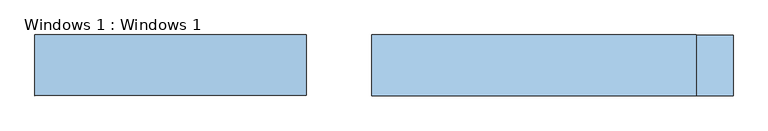
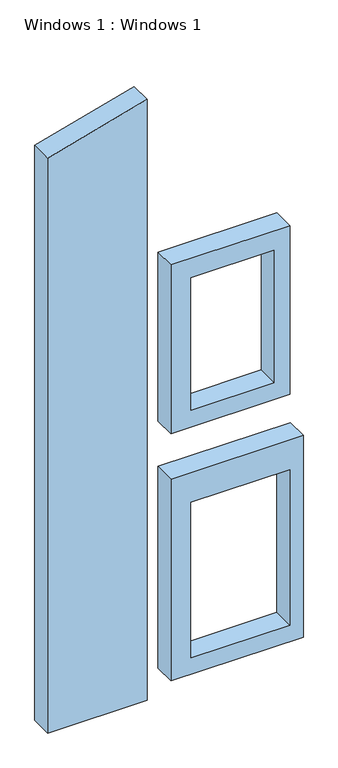
"""IFC4 building model written with IfcOpenShell, lengths in millimetres: window geometry, Windows 1 : Windows 1."""

from ifc_helpers import new_model, si_unit, point, frame, frame_2d, origin, place, context, project, spatial, polyline, circle_curve, trimmed, segment, composite_curve, outline, extrude, source, transform, mapped, element, save


def windows_1_windows_1_253e0c66(model_context):
    return source(origin(), model_context, "Body", "SweptSolid", [
        extrude(outline(composite_curve([segment(polyline([(-400.0, -18502.079547), (-400.0, -15162.2234094), (20949.827623, -15162.2234094)]), True, "CONTINUOUS"), segment(trimmed(circle_curve(frame_2d((-3469.7681282, -10237.7954873)), 24911.1751431), [point((20949.827623, -15162.2234094))], [point((20030.620294, -18502.079547))], False, "CARTESIAN"), True, "CONTINUOUS"), segment(polyline([(20030.620294, -18502.079547), (-400.0, -18502.079547)]), True, "CONTINUOUS")], self_intersect=False)), frame((0.0, -11139.4093514, 0.0), z_axis=(0.0, 1.0, 0.0), x_axis=(0.0, 0.0, 1.0)), (0.0, 0.0, 1.0), 746.1893999),
        extrude(outline(polyline([(8784.7000326, -14354.7304495), (8784.7000326, -10354.7304495), (14784.7000326, -10354.7304495), (14784.7000326, -14354.7304495), (8784.7000326, -14354.7304495)]), holes=[polyline([(9386.7117588, -13683.063222), (14086.7117588, -13683.063222), (14086.7117588, -10883.063222), (9386.7117588, -10883.063222), (9386.7117588, -13683.063222)])]), frame((0.0, -11139.4093514, 0.0), z_axis=(0.0, 1.0, 0.0), x_axis=(0.0, 0.0, 1.0)), (0.0, 0.0, 1.0), 746.1893999),
        extrude(outline(polyline([(0.0, -14354.7304495), (0.0, -9902.079547), (7173.1778584, -9902.079547), (7173.1778584, -14354.7304495), (0.0, -14354.7304495)]), holes=[polyline([(581.6088758, -13683.063222), (6108.2161014, -13683.063222), (6108.2161014, -10354.7304495), (581.6088758, -10354.7304495), (581.6088758, -13683.063222)])]), frame((0.0, -11139.4093514, 0.0), z_axis=(0.0, 1.0, 0.0), x_axis=(0.0, 0.0, 1.0)), (0.0, 0.0, 1.0), 746.1893999),
    ])


if __name__ == "__main__":
    model = new_model("IFC4")
    model_context = context("Model", 3, world=origin())
    ifc_project = project(units=[si_unit("LENGTHUNIT", "METRE", prefix="MILLI")], contexts=[model_context])
    site = spatial("IfcSite", under=ifc_project)
    building = spatial("IfcBuilding", under=site)
    placement = place(None, origin())
    windows_1_windows_1_shape = windows_1_windows_1_253e0c66(model_context)
    element("IfcWindow", 1, ObjectType="Windows 1 : Windows 1", at=placement, inside=building, context=model_context, shape_type="MappedRepresentation", body=[
        mapped(windows_1_windows_1_shape, transform((0.0, 0.0, 0.0), x_axis=(1.0, 0.0, 0.0), y_axis=(0.0, 1.0, 0.0), z_axis=(0.0, 0.0, 1.0))),
    ])
    save(model, "model.ifc")

# Revit data of these elements
# Type "Windows 1 : Windows 1"
#   Type Mark = "24"
